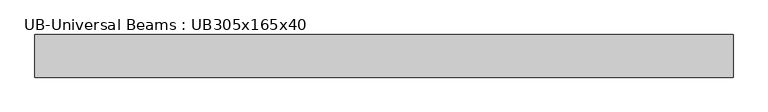
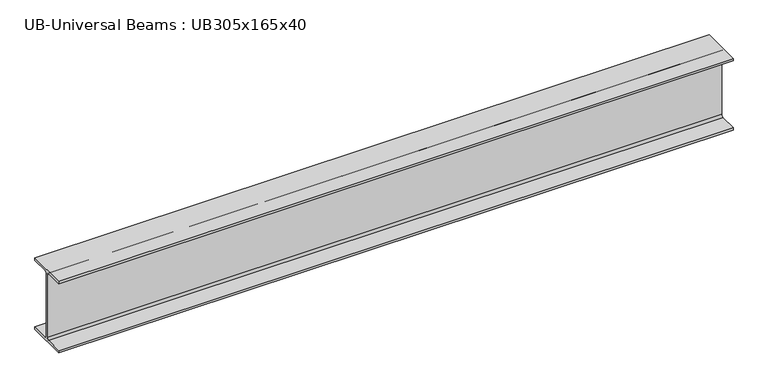
"""IFC4 building model written with IfcOpenShell, lengths in millimetres: beam geometry, UB-Universal Beams : UB305x165x40."""

from ifc_helpers import new_model, si_unit, point, frame, frame_2d, origin, place, context, project, spatial, polyline, circle_curve, trimmed, segment, composite_curve, outline, extrude, source, transform, mapped, element, save


def ub_universal_beams_ub305x165x40_6c2df09e(model_context):
    return source(origin(), model_context, "Body", "SweptSolid", [
        extrude(outline(composite_curve([segment(polyline([(82.5, -141.5), (82.5, -151.7), (-82.5, -151.7), (-82.5, -141.5), (-11.9, -141.5)]), True, "CONTINUOUS"), segment(trimmed(circle_curve(frame_2d((-11.9, -132.6)), 8.9), [point((-11.9, -141.5))], [point((-3.0, -132.6))], True, "CARTESIAN"), True, "CONTINUOUS"), segment(polyline([(-3.0, -132.6), (-3.0, 132.6)]), True, "CONTINUOUS"), segment(trimmed(circle_curve(frame_2d((-11.9, 132.6)), 8.9), [point((-3.0, 132.6))], [point((-11.9, 141.5))], True, "CARTESIAN"), True, "CONTINUOUS"), segment(polyline([(-11.9, 141.5), (-82.5, 141.5), (-82.5, 151.7), (82.5, 151.7), (82.5, 141.5), (11.9, 141.5)]), True, "CONTINUOUS"), segment(trimmed(circle_curve(frame_2d((11.9, 132.6)), 8.9), [point((11.9, 141.5))], [point((3.0, 132.6))], True, "CARTESIAN"), True, "CONTINUOUS"), segment(polyline([(3.0, 132.6), (3.0, -132.6)]), True, "CONTINUOUS"), segment(trimmed(circle_curve(frame_2d((11.9, -132.6)), 8.9), [point((3.0, -132.6))], [point((11.9, -141.5))], True, "CARTESIAN"), True, "CONTINUOUS"), segment(polyline([(11.9, -141.5), (82.5, -141.5)]), True, "CONTINUOUS")], self_intersect=False)), frame((-1401.6, 0.0, 0.0), z_axis=(1.0, 0.0, 0.0), x_axis=(0.0, 1.0, 0.0)), (0.0, 0.0, 1.0), 2703.9),
    ])


if __name__ == "__main__":
    model = new_model("IFC4")
    model_context = context("Model", 3, world=origin())
    ifc_project = project(units=[si_unit("LENGTHUNIT", "METRE", prefix="MILLI")], contexts=[model_context])
    site = spatial("IfcSite", under=ifc_project)
    building = spatial("IfcBuilding", under=site)
    placement = place(None, origin())
    ub_universal_beams_ub305x165x40_shape = ub_universal_beams_ub305x165x40_6c2df09e(model_context)
    element("IfcBeam", 1, ObjectType="UB-Universal Beams : UB305x165x40", at=placement, inside=building, context=model_context, shape_type="MappedRepresentation", body=[
        mapped(ub_universal_beams_ub305x165x40_shape, transform((0.0, 0.0, 0.0), x_axis=(1.0, 0.0, 0.0), y_axis=(0.0, 1.0, 0.0), z_axis=(0.0, 0.0, 1.0))),
    ])
    save(model, "model.ifc")

# Revit data of these elements
# Type "UB-Universal Beams : UB305x165x40"
#   Section Name Key = "UB305X165X40"
#   Width = 16.5 cm
#   Web Thickness = 0.6 cm
#   Web Fillet = 0.89 cm
#   Warping Constant = 164000.0 cm⁶
#   Torsional Moment of Inertia = 14.70 cm⁴
#   Section Area = 51.3 cm²
#   Plastic Modulus weak axis = 142.0 cm³
#   Plastic Modulus strong axis = 623.0 cm³
#   Nominal Weight = 40.2999 kgf/m
#   Moment of Inertia weak axis = 764.00 cm⁴
#   Moment of Inertia strong axis = 8503.00 cm⁴
#   Height = 30.34 cm
#   Flange Thickness = 1.02 cm
#   Elastic Modulus weak axis = 92.6 cm³
#   Elastic Modulus strong axis = 560.0 cm³
#   Centroid Vertical = 15.17 cm
#   Centroid Horizontal = 8.25 cm
#   Bolt Spacing = 9.0 cm
#   Length [instance default] = 1500 mm
#   Structural Material [instance default] = Metal - Steel 43-275
#   Type Comments = ""
#   Assembly Code = ""
# Element 1 (IfcBeam, "UB-Universal Beams : UB305x165x40")
#   Materials on its faces: "Metal - Steel 43-275"
# Materials
#   "Metal - Steel 43-275": class "Metal", colour RGB 247 247 247, transparency 0, Cost = 0
